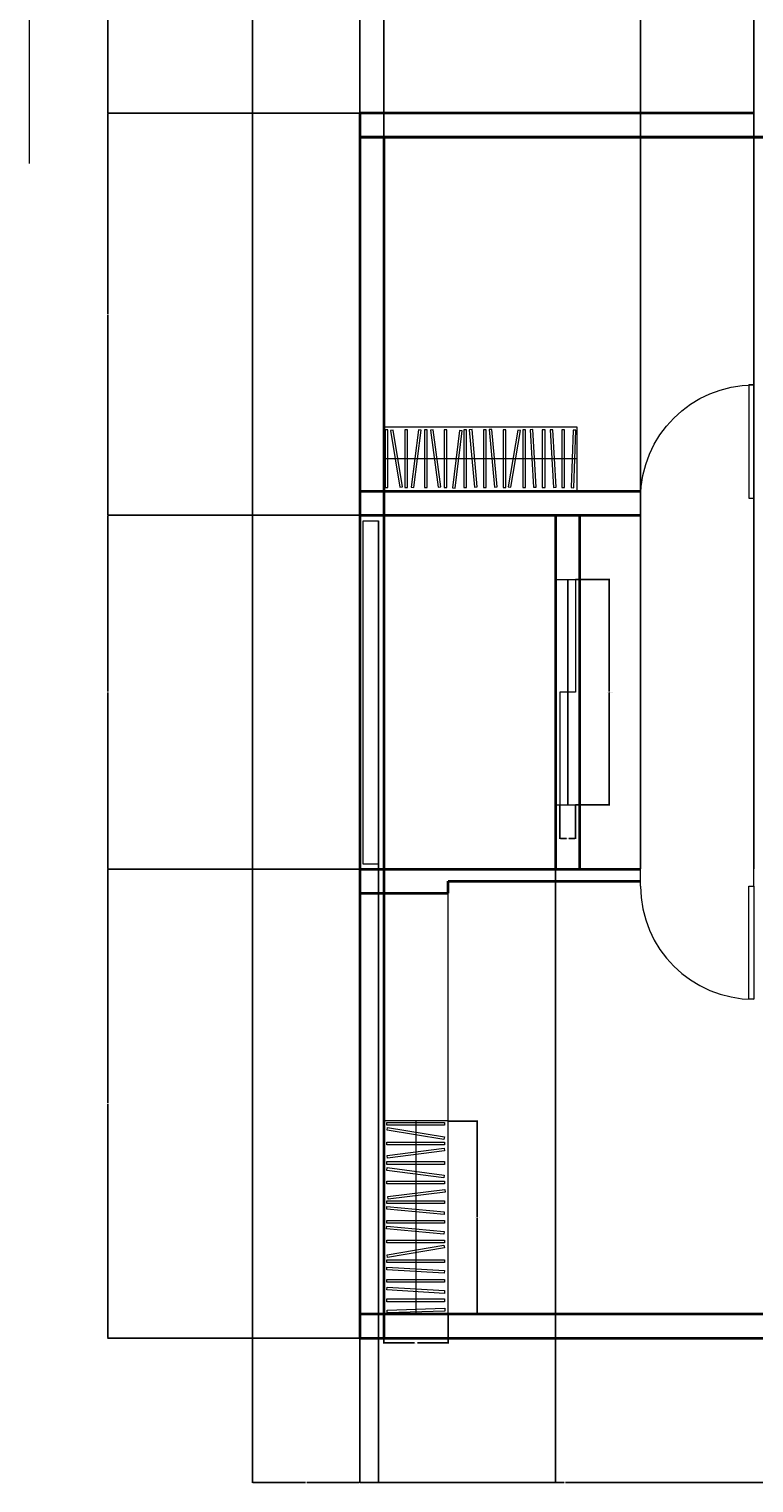
# Model space of a CAD drawing. Units: inches. Extents: x 531915 to 533151, y 849859 to 851471.
# Tile 2 of 7: x 531939 to 532210, y 850315 to 850858. Entities that reach past the tile are written whole.
import ezdxf

# ---------------------------------------------------------------- set-up
doc = ezdxf.new("R2010")
doc.units = ezdxf.units.IN
for name, color, linetype, lineweight in [('A-ANNO-DIMS', 2, 'Continuous', 18), ('A-DOOR', 3, 'Continuous', 18), ('A-FLOR-HRAL', 4, 'Continuous', 20), ('A-FURN', 8, 'Continuous', 13), ('A-WALL', 7, 'Continuous', 35)]:
    doc.layers.add(name, color=color, linetype=linetype, lineweight=lineweight)
doc.styles.get("Standard").update_dxf_attribs({"font": 'arial.ttf'})
doc.dimstyles.get("Standard").update_dxf_attribs({"dimtxt": 0.18, "dimasz": 0.18, "dimexe": 0.18, "dimexo": 0.0625, "dimgap": 0.09, "dimtad": 0, "dimtih": 1, "dimtoh": 1, "dimdec": 4, "dimzin": 0, "dimdsep": 46, "dimtxsty": 'Standard', "dimcen": 0.09, "dimadec": 0, "dimazin": 0, "dimtfac": 1, "dimtdec": 4, "dimtofl": 0, "dimtmove": 0, "dimatfit": 3, "dimfxl": 1, "dimtolj": 1, "dimtzin": 0, "dimarcsym": 0})

# ---------------------------------------------------------------- blocks, each defined once
blk = doc.blocks.new('*U2')
for p, q in [((0, 0), (0, -6)), ((40, 0), (40, -6))]:
    blk.add_line(p, q)
blk.add_lwpolyline([(0, 0), (0, 40), (1.75, 40), (1.75, 0)], close=True)
blk.add_arc((0, 0), 40, 0, 90)
blk = doc.blocks.new('WARDROBE-72')
blk.add_line((12, 0), (12, 72))
for points in [[(24, 0), (24, 72), (0, 72), (0, 0)], [(1.15, 70.47), (1.15, 71.48), (22.64, 71.48), (22.64, 70.47)], [(1.21, 68.56), (1.37, 69.55), (22.58, 66.07), (22.41, 65.07)], [(1.15, 63.15), (1.15, 64.16), (22.64, 64.16), (22.64, 63.15)], [(1.3, 58.13), (1.17, 59.13), (22.48, 61.86), (22.61, 60.86)], [(1.11, 53.59), (1.24, 54.59), (22.54, 51.79), (22.41, 50.79)], [(1.15, 55.83), (1.15, 56.84), (22.64, 56.84), (22.64, 55.83)], [(1.15, 48.51), (1.15, 49.52), (22.64, 49.52), (22.64, 48.51)], [(1.55, 42.84), (1.42, 43.84), (22.76, 46.42), (22.88, 45.42)], [(1.04, 39.13), (1.13, 40.14), (22.52, 38.16), (22.43, 37.15)], [(1.15, 41.19), (1.15, 42.2), (22.64, 42.2), (22.64, 41.19)], [(0.98, 31.76), (1.07, 32.76), (22.47, 30.78), (22.37, 29.78)], [(1.15, 33.87), (1.15, 34.88), (22.64, 34.88), (22.64, 33.87)], [(1.15, 26.55), (1.15, 27.56), (22.64, 27.56), (22.64, 26.55)], [(1.38, 21.1), (1.21, 22.1), (22.4, 25.68), (22.57, 24.68)], [(1.05, 16.46), (1.11, 17.47), (22.56, 16.21), (22.5, 15.2)], [(1.15, 19.23), (1.15, 20.24), (22.64, 20.24), (22.64, 19.23)], [(1.15, 11.91), (1.15, 12.92), (22.64, 12.92), (22.64, 11.91)], [(1.11, 8.97), (1.17, 9.98), (22.62, 8.71), (22.56, 7.7)], [(1.15, 4.59), (1.15, 5.6), (22.64, 5.6), (22.64, 4.59)], [(1.25, 0.42), (1.22, 1.43), (22.7, 2.11), (22.73, 1.1)]]:
    blk.add_lwpolyline(points, close=True)
blk = doc.blocks.new('BALCONY-SLIDER-84')
blk.add_line((2.88, 84), (2.88, 0))
for points in [[(2.88, 84), (5.76, 84), (5.76, 41.94), (2.88, 41.94)], [(2.88, 41.94), (0, 41.94), (0, 0), (2.88, 0)]]:
    blk.add_lwpolyline(points, close=True)
blk = doc.blocks.new('*D15')
at = {"layer": 'A-ANNO-DIMS', "color": 0, "lineweight": -2, "transparency": 16777216}
for p, q in [((532095.87, 850450.37), (532106.78, 850450.37)), ((532106.6, 850450.19), (532106.6, 850414.56)), ((532106.6, 850378.55), (532106.6, 850414.19)), ((532095.87, 850378.37), (532106.78, 850378.37))]:
    blk.add_line(p, q, dxfattribs=at)
at = {"layer": 'A-ANNO-DIMS', "color": 0, "transparency": 16777216}
for points in [[(532106.57, 850450.19), (532106.63, 850450.19), (532106.6, 850450.37)], [(532106.57, 850378.55), (532106.63, 850378.55), (532106.6, 850378.37)]]:
    blk.add_solid(points, dxfattribs=at)
at = {"layer": 'Defpoints', "color": 0, "transparency": 16777216}
for p in [(532095.8, 850450.37), (532106.6, 850450.37), (532095.8, 850378.37)]:
    blk.add_point(p, dxfattribs=at)
at = {"layer": 'A-ANNO-DIMS', "color": 0, "transparency": 16777216, "insert": (532106.6, 850414.37), "char_height": 0.18, "attachment_point": 5}
blk.add_mtext('\\A1;WARDROBE 72 TYP.', dxfattribs=at)
blk = doc.blocks.new('*D16')
at = {"layer": 'A-ANNO-DIMS', "color": 0, "lineweight": -2, "transparency": 16777216}
for p, q in [((532071.8, 850378.31), (532071.8, 850367.39)), ((532095.8, 850378.31), (532095.8, 850367.39)), ((532071.98, 850367.57), (532083.28, 850367.57)), ((532095.62, 850367.57), (532084.33, 850367.57))]:
    blk.add_line(p, q, dxfattribs=at)
at = {"layer": 'A-ANNO-DIMS', "color": 0, "transparency": 16777216}
for points in [[(532071.98, 850367.6), (532071.98, 850367.54), (532071.8, 850367.57)], [(532095.62, 850367.6), (532095.62, 850367.54), (532095.8, 850367.57)]]:
    blk.add_solid(points, dxfattribs=at)
at = {"layer": 'Defpoints', "color": 0, "transparency": 16777216}
for p in [(532071.8, 850378.37), (532095.8, 850378.37), (532095.8, 850367.57)]:
    blk.add_point(p, dxfattribs=at)
at = {"layer": 'A-ANNO-DIMS', "color": 0, "transparency": 16777216, "insert": (532083.8, 850367.57), "char_height": 0.18, "attachment_point": 5}
blk.add_mtext('\\A1;24 TYP.', dxfattribs=at)
blk = doc.blocks.new('*D29')
at = {"layer": 'A-ANNO-DIMS', "color": 0, "lineweight": -2, "transparency": 16777216}
for p, q in [((532143.29, 850652.37), (532156.01, 850652.37)), ((532155.83, 850652.19), (532155.83, 850610.56)), ((532155.83, 850568.55), (532155.83, 850610.19)), ((532143.29, 850568.37), (532156.01, 850568.37))]:
    blk.add_line(p, q, dxfattribs=at)
at = {"layer": 'A-ANNO-DIMS', "color": 0, "transparency": 16777216}
for points in [[(532155.8, 850652.19), (532155.86, 850652.19), (532155.83, 850652.37)], [(532155.8, 850568.55), (532155.86, 850568.55), (532155.83, 850568.37)]]:
    blk.add_solid(points, dxfattribs=at)
at = {"layer": 'Defpoints', "color": 0, "transparency": 16777216}
for p in [(532143.23, 850652.37), (532155.83, 850652.37), (532143.23, 850568.37)]:
    blk.add_point(p, dxfattribs=at)
at = {"layer": 'A-ANNO-DIMS', "color": 0, "transparency": 16777216, "insert": (532155.83, 850610.37), "char_height": 0.18, "attachment_point": 5}
blk.add_mtext('\\A1;BALCONY SLIDER 84 TYP.', dxfattribs=at)
blk = doc.blocks.new('*D30')
at = {"layer": 'A-ANNO-DIMS', "color": 0, "lineweight": -2, "transparency": 16777216}
for p, q in [((532137.47, 850568.31), (532137.47, 850555.59)), ((532143.23, 850568.31), (532143.23, 850555.59)), ((532137.65, 850555.77), (532139.89, 850555.77)), ((532143.05, 850555.77), (532140.81, 850555.77))]:
    blk.add_line(p, q, dxfattribs=at)
at = {"layer": 'A-ANNO-DIMS', "color": 0, "transparency": 16777216}
for points in [[(532137.65, 850555.8), (532137.65, 850555.74), (532137.47, 850555.77)], [(532143.05, 850555.8), (532143.05, 850555.74), (532143.23, 850555.77)]]:
    blk.add_solid(points, dxfattribs=at)
at = {"layer": 'Defpoints', "color": 0, "transparency": 16777216}
for p in [(532137.47, 850568.37), (532143.23, 850568.37), (532143.23, 850555.77)]:
    blk.add_point(p, dxfattribs=at)
at = {"layer": 'A-ANNO-DIMS', "color": 0, "transparency": 16777216, "insert": (532140.35, 850555.77), "char_height": 0.18, "attachment_point": 5}
blk.add_mtext('\\A1;6 TYP.', dxfattribs=at)
blk = doc.blocks.new('*D41')
at = {"layer": 'A-ANNO-DIMS', "color": 0, "lineweight": -2, "transparency": 16777216}
for p, q in [((532451.74, 850922.23), (531968.71, 850922.23)), ((531968.89, 850922.05), (531968.89, 850874.49)), ((531968.89, 850826.55), (531968.89, 850874.12)), ((532062.74, 850826.37), (531968.71, 850826.37))]:
    blk.add_line(p, q, dxfattribs=at)
at = {"layer": 'A-ANNO-DIMS', "color": 0, "transparency": 16777216}
for points in [[(531968.86, 850922.05), (531968.92, 850922.05), (531968.89, 850922.23)], [(531968.86, 850826.55), (531968.92, 850826.55), (531968.89, 850826.37)]]:
    blk.add_solid(points, dxfattribs=at)
at = {"layer": 'Defpoints', "color": 0, "transparency": 16777216}
for p in [(532451.8, 850922.23), (531968.89, 850826.37), (532062.8, 850826.37)]:
    blk.add_point(p, dxfattribs=at)
at = {"layer": 'A-ANNO-DIMS', "color": 0, "transparency": 16777216, "insert": (531968.89, 850874.3), "char_height": 0.18, "attachment_point": 5}
blk.add_mtext('\\A1;95.86', dxfattribs=at)
blk = doc.blocks.new('*D46')
at = {"layer": 'A-ANNO-DIMS', "color": 0, "lineweight": -2, "transparency": 16777216}
for p, q in [((532022.8, 850946.31), (532022.8, 850315.34)), ((532062.8, 850826.31), (532062.8, 850315.34)), ((532022.98, 850315.52), (532042.58, 850315.52)), ((532062.62, 850315.52), (532043.03, 850315.52))]:
    blk.add_line(p, q, dxfattribs=at)
at = {"layer": 'A-ANNO-DIMS', "color": 0, "transparency": 16777216}
for points in [[(532022.98, 850315.55), (532022.98, 850315.49), (532022.8, 850315.52)], [(532062.62, 850315.55), (532062.62, 850315.49), (532062.8, 850315.52)]]:
    blk.add_solid(points, dxfattribs=at)
at = {"layer": 'Defpoints', "color": 0, "transparency": 16777216}
for p in [(532022.8, 850946.37), (532062.8, 850826.37), (532062.8, 850315.52)]:
    blk.add_point(p, dxfattribs=at)
at = {"layer": 'A-ANNO-DIMS', "color": 0, "transparency": 16777216, "insert": (532042.8, 850315.52), "char_height": 0.18, "attachment_point": 5}
blk.add_mtext('\\A1;40', dxfattribs=at)
blk = doc.blocks.new('*D60')
at = {"layer": 'A-ANNO-DIMS', "color": 0, "lineweight": -2, "transparency": 16777216}
for p, q in [((532062.8, 850369.31), (532062.8, 850315.34)), ((532215.8, 850369.31), (532215.8, 850315.34)), ((532062.98, 850315.52), (532139.02, 850315.52)), ((532215.62, 850315.52), (532139.59, 850315.52))]:
    blk.add_line(p, q, dxfattribs=at)
at = {"layer": 'A-ANNO-DIMS', "color": 0, "transparency": 16777216}
for points in [[(532062.98, 850315.55), (532062.98, 850315.49), (532062.8, 850315.52)], [(532215.62, 850315.55), (532215.62, 850315.49), (532215.8, 850315.52)]]:
    blk.add_solid(points, dxfattribs=at)
at = {"layer": 'Defpoints', "color": 0, "transparency": 16777216}
for p in [(532062.8, 850369.37), (532215.8, 850369.37), (532215.8, 850315.52)]:
    blk.add_point(p, dxfattribs=at)
at = {"layer": 'A-ANNO-DIMS', "color": 0, "transparency": 16777216, "insert": (532139.3, 850315.52), "char_height": 0.18, "attachment_point": 5}
blk.add_mtext('\\A1;153', dxfattribs=at)
blk = doc.blocks.new('*D63')
at = {"layer": 'A-ANNO-DIMS', "color": 0, "lineweight": -2, "transparency": 16777216}
for p, q in [((532062.74, 850826.37), (531968.71, 850826.37)), ((531968.89, 850826.19), (531968.89, 850751.56)), ((531968.89, 850676.55), (531968.89, 850751.19)), ((532062.74, 850676.37), (531968.71, 850676.37))]:
    blk.add_line(p, q, dxfattribs=at)
at = {"layer": 'A-ANNO-DIMS', "color": 0, "transparency": 16777216}
for points in [[(531968.86, 850826.19), (531968.92, 850826.19), (531968.89, 850826.37)], [(531968.86, 850676.55), (531968.92, 850676.55), (531968.89, 850676.37)]]:
    blk.add_solid(points, dxfattribs=at)
at = {"layer": 'Defpoints', "color": 0, "transparency": 16777216}
for p in [(532062.8, 850826.37), (531968.89, 850676.37), (532062.8, 850676.37)]:
    blk.add_point(p, dxfattribs=at)
at = {"layer": 'A-ANNO-DIMS', "color": 0, "transparency": 16777216, "insert": (531968.89, 850751.37), "char_height": 0.18, "attachment_point": 5}
blk.add_mtext('\\A1;150', dxfattribs=at)
blk = doc.blocks.new('*D64')
at = {"layer": 'A-ANNO-DIMS', "color": 0, "lineweight": -2, "transparency": 16777216}
for p, q in [((532062.74, 850676.37), (531968.71, 850676.37)), ((531968.89, 850676.19), (531968.89, 850610.56)), ((531968.89, 850544.55), (531968.89, 850610.19)), ((532062.74, 850544.37), (531968.71, 850544.37))]:
    blk.add_line(p, q, dxfattribs=at)
at = {"layer": 'A-ANNO-DIMS', "color": 0, "transparency": 16777216}
for points in [[(531968.86, 850676.19), (531968.92, 850676.19), (531968.89, 850676.37)], [(531968.86, 850544.55), (531968.92, 850544.55), (531968.89, 850544.37)]]:
    blk.add_solid(points, dxfattribs=at)
at = {"layer": 'Defpoints', "color": 0, "transparency": 16777216}
for p in [(532062.8, 850676.37), (531968.89, 850544.37), (532062.8, 850544.37)]:
    blk.add_point(p, dxfattribs=at)
at = {"layer": 'A-ANNO-DIMS', "color": 0, "transparency": 16777216, "insert": (531968.89, 850610.37), "char_height": 0.18, "attachment_point": 5}
blk.add_mtext('\\A1;132', dxfattribs=at)
blk = doc.blocks.new('*D65')
at = {"layer": 'A-ANNO-DIMS', "color": 0, "lineweight": -2, "transparency": 16777216}
for p, q in [((532062.74, 850544.37), (531968.71, 850544.37)), ((531968.89, 850544.19), (531968.89, 850457.06)), ((531968.89, 850369.55), (531968.89, 850456.69)), ((532062.74, 850369.37), (531968.71, 850369.37))]:
    blk.add_line(p, q, dxfattribs=at)
at = {"layer": 'A-ANNO-DIMS', "color": 0, "transparency": 16777216}
for points in [[(531968.86, 850544.19), (531968.92, 850544.19), (531968.89, 850544.37)], [(531968.86, 850369.55), (531968.92, 850369.55), (531968.89, 850369.37)]]:
    blk.add_solid(points, dxfattribs=at)
at = {"layer": 'Defpoints', "color": 0, "transparency": 16777216}
for p in [(532062.8, 850544.37), (531968.89, 850369.37), (532062.8, 850369.37)]:
    blk.add_point(p, dxfattribs=at)
at = {"layer": 'A-ANNO-DIMS', "color": 0, "transparency": 16777216, "insert": (531968.89, 850456.87), "char_height": 0.18, "attachment_point": 5}
blk.add_mtext('\\A1;175', dxfattribs=at)
blk = doc.blocks.new('*D66')
at = {"layer": 'A-ANNO-DIMS', "color": 0, "lineweight": -2, "transparency": 16777216}
for p, q in [((532135.8, 850676.31), (532135.8, 850315.34)), ((532069.82, 850674.18), (532069.82, 850315.34)), ((532070, 850315.52), (532102.42, 850315.52)), ((532135.62, 850315.52), (532103.21, 850315.52))]:
    blk.add_line(p, q, dxfattribs=at)
at = {"layer": 'A-ANNO-DIMS', "color": 0, "transparency": 16777216}
for points in [[(532070, 850315.55), (532070, 850315.49), (532069.82, 850315.52)], [(532135.62, 850315.55), (532135.62, 850315.49), (532135.8, 850315.52)]]:
    blk.add_solid(points, dxfattribs=at)
at = {"layer": 'Defpoints', "color": 0, "transparency": 16777216}
for p in [(532135.8, 850676.37), (532069.82, 850674.24), (532135.8, 850315.52)]:
    blk.add_point(p, dxfattribs=at)
at = {"layer": 'A-ANNO-DIMS', "color": 0, "transparency": 16777216, "insert": (532102.81, 850315.52), "char_height": 0.18, "attachment_point": 5}
blk.add_mtext('\\A1;65.98', dxfattribs=at)
blk = doc.blocks.new('*D81')
at = {"layer": 'A-ANNO-DIMS', "color": 0, "lineweight": -2, "transparency": 16777216}
for p, q in [((532062.8, 850826.44), (532062.8, 851470.96)), ((532062.98, 851470.78), (532067.16, 851470.78)), ((532071.62, 851470.78), (532067.45, 851470.78)), ((532071.8, 850817.44), (532071.8, 851470.96))]:
    blk.add_line(p, q, dxfattribs=at)
at = {"layer": 'A-ANNO-DIMS', "color": 0, "transparency": 16777216}
for points in [[(532062.98, 851470.81), (532062.98, 851470.75), (532062.8, 851470.78)], [(532071.62, 851470.81), (532071.62, 851470.75), (532071.8, 851470.78)]]:
    blk.add_solid(points, dxfattribs=at)
at = {"layer": 'Defpoints', "color": 0, "transparency": 16777216}
for p in [(532071.8, 851470.78), (532062.8, 850826.37), (532071.8, 850817.37)]:
    blk.add_point(p, dxfattribs=at)
at = {"layer": 'A-ANNO-DIMS', "color": 0, "transparency": 16777216, "insert": (532067.3, 851470.78), "char_height": 0.18, "attachment_point": 5}
blk.add_mtext('\\A1;9', dxfattribs=at)
blk = doc.blocks.new('*D86')
at = {"layer": 'A-ANNO-DIMS', "color": 0, "lineweight": -2, "transparency": 16777216}
for p, q in [((532167.55, 850544.44), (532167.55, 851470.96)), ((532167.73, 851470.78), (532188.28, 851470.78)), ((532209.62, 851470.78), (532189.08, 851470.78)), ((532209.8, 850544.44), (532209.8, 851470.96))]:
    blk.add_line(p, q, dxfattribs=at)
at = {"layer": 'A-ANNO-DIMS', "color": 0, "transparency": 16777216}
for points in [[(532167.73, 851470.81), (532167.73, 851470.75), (532167.55, 851470.78)], [(532209.62, 851470.81), (532209.62, 851470.75), (532209.8, 851470.78)]]:
    blk.add_solid(points, dxfattribs=at)
at = {"layer": 'Defpoints', "color": 0, "transparency": 16777216}
for p in [(532209.8, 851470.78), (532167.55, 850544.37), (532209.8, 850544.37)]:
    blk.add_point(p, dxfattribs=at)
at = {"layer": 'A-ANNO-DIMS', "color": 0, "transparency": 16777216, "insert": (532188.68, 851470.78), "char_height": 0.18, "attachment_point": 5}
blk.add_mtext('\\A1;42.25', dxfattribs=at)

msp = doc.modelspace()

# ---------------------------------------------------------------- linework, layer by layer
at = {"layer": 'A-DOOR'}
for p, q in [((532135.8048, 850652.374), (532144.8048, 850652.374)), ((532135.8048, 850568.374), (532144.8048, 850568.374))]:
    msp.add_line(p, q, dxfattribs=at)
at = {"layer": 'A-FLOR-HRAL'}
msp.add_lwpolyline([(532064.0957, 850674.239), (532069.8248, 850674.239), (532069.8248, 850546.2421), (532064.0957, 850546.2421)], close=True, dxfattribs=at)
at = {"layer": 'A-FURN'}
for p, q in [((531939.4832, 850892.5471), (531939.4832, 850807.5471)), ((532095.8048, 850450.374), (532095.8048, 850535.374))]:
    msp.add_line(p, q, dxfattribs=at)
at = {"layer": 'A-WALL'}
for p, q in [((532062.8048, 850826.374), (532062.8048, 850369.374)), ((532209.8048, 850826.374), (532062.8048, 850826.374)), ((532442.8048, 850817.374), (532062.8048, 850817.374)), ((532062.8048, 850817.374), (532451.8048, 850817.374)), ((532071.8048, 850817.374), (532071.8048, 850369.374)), ((532062.8048, 850685.374), (532167.637, 850685.374)), ((532062.8048, 850676.374), (532167.553, 850676.374)), ((532135.8048, 850676.374), (532135.8048, 850544.374)), ((532144.8048, 850676.374), (532144.8048, 850544.374)), ((532062.8048, 850544.374), (532167.553, 850544.374)), ((532095.8048, 850535.374), (532095.8048, 850539.874)), ((532095.8048, 850539.874), (532167.553, 850539.874)), ((532062.8048, 850535.374), (532095.8048, 850535.374)), ((532071.8048, 850535.374), (532095.8048, 850535.374)), ((532062.8048, 850378.374), (532676.8048, 850378.374)), ((532062.8048, 850369.374), (532676.8048, 850369.374))]:
    msp.add_line(p, q, dxfattribs=at)

# ---------------------------------------------------------------- block references
at = {"layer": 'A-DOOR', "xscale": -1.056294156906435, "yscale": 1.056294156906435, "zscale": 1.056294156906435}
msp.add_blockref('*U2', (532209.8048, 850682.7117), dxfattribs=at)
at = {"layer": 'A-DOOR'}
msp.add_blockref('BALCONY-SLIDER-84', (532137.4675, 850568.374), dxfattribs=at)
at = {"layer": 'A-DOOR', "xscale": 1.056294156906435, "yscale": 1.056294156906435, "zscale": 1.056294156906435, "rotation": 180}
msp.add_blockref('*U2', (532209.8048, 850538.0362), dxfattribs=at)
at = {"layer": 'A-FURN', "extrusion": (0, 0, -1), "zscale": -1, "rotation": 269.9999999995917}
msp.add_blockref('WARDROBE-72', (-532143.8048, 850709.374), dxfattribs=at)
at = {"layer": 'A-FURN'}
msp.add_blockref('WARDROBE-72', (532071.8048, 850378.374), dxfattribs=at)

# ---------------------------------------------------------------- dimensions: what is measured, and where the dimension line sits
at = {"layer": 'A-ANNO-DIMS'}
for base, p1, p2, override, picture, middle in [((532071.8048, 851470.7848), (532062.8048, 850826.374), (532071.8048, 850817.374), {"dimdec": 0, "dimlfac": 1, "dimrnd": 0, "dimzin": 0, "dimdsep": 46, "dimlunit": 2}, '*D81', (532067.3048, 851470.7848)), ((532209.8048, 851470.7848), (532167.553, 850544.374), (532209.8048, 850544.374), {"dimdec": 2, "dimlfac": 1, "dimrnd": 0, "dimzin": 0, "dimdsep": 46, "dimlunit": 2}, '*D86', (532188.6789, 851470.7848)), ((532062.8048, 850315.524), (532022.8048, 850946.374), (532062.8048, 850826.374), {"dimdec": 0, "dimlfac": 1, "dimrnd": 0, "dimzin": 0, "dimdsep": 46, "dimlunit": 2}, '*D46', (532042.8048, 850315.524)), ((532135.8048, 850315.524), (532069.8248, 850674.239), (532135.8048, 850676.374), {"dimdec": 2, "dimlfac": 1, "dimrnd": 0, "dimzin": 0, "dimdsep": 46, "dimlunit": 2}, '*D66', (532102.8148, 850315.524)), ((532215.8048, 850315.524), (532062.8048, 850369.374), (532215.8048, 850369.374), {"dimdec": 0, "dimlfac": 1, "dimrnd": 0, "dimzin": 0, "dimdsep": 46, "dimlunit": 2}, '*D60', (532139.3048, 850315.524))]:
    dim = msp.add_linear_dim(base=base, p1=p1, p2=p2, dimstyle='Standard', override=override, dxfattribs=at)
    dim.commit()
    dim.dimension.update_dxf_attribs({"geometry": picture, "text_midpoint": middle})
for base, p1, p2, override, picture, middle in [((531968.8939, 850826.374), (532451.8048, 850922.2344), (532062.8048, 850826.374), {"dimdec": 2, "dimlfac": 1, "dimrnd": 0, "dimzin": 0, "dimdsep": 46, "dimlunit": 2}, '*D41', (531968.8939, 850874.3042)), ((531968.8939, 850676.374), (532062.8048, 850826.374), (532062.8048, 850676.374), {"dimdec": 0, "dimlfac": 1, "dimrnd": 0, "dimzin": 0, "dimdsep": 46, "dimlunit": 2}, '*D63', (531968.8939, 850751.374)), ((531968.8939, 850544.374), (532062.8048, 850676.374), (532062.8048, 850544.374), {"dimdec": 0, "dimlfac": 1, "dimrnd": 0, "dimzin": 0, "dimdsep": 46, "dimlunit": 2}, '*D64', (531968.8939, 850610.374)), ((531968.8939, 850369.374), (532062.8048, 850544.374), (532062.8048, 850369.374), {"dimdec": 0, "dimlfac": 1, "dimrnd": 0, "dimzin": 0, "dimdsep": 46, "dimlunit": 2}, '*D65', (531968.8939, 850456.874))]:
    dim = msp.add_linear_dim(base=base, p1=p1, p2=p2, angle=90, dimstyle='Standard', override=override, dxfattribs=at)
    dim.commit()
    dim.dimension.update_dxf_attribs({"geometry": picture, "text_midpoint": middle})
for base, p1, p2, text, picture, middle in [((532155.8316, 850652.374), (532143.2316, 850568.374), (532143.2316, 850652.374), 'BALCONY SLIDER <> TYP.', '*D29', (532155.8316, 850610.374)), ((532106.6048, 850450.374), (532095.8048, 850378.374), (532095.8048, 850450.374), 'WARDROBE <> TYP.', '*D15', (532106.6048, 850414.374))]:
    dim = msp.add_linear_dim(base=base, p1=p1, p2=p2, angle=90, text=text, dimstyle='Standard', override={"dimdec": 0, "dimlfac": 1, "dimrnd": 0, "dimzin": 0, "dimdsep": 46, "dimlunit": 2}, dxfattribs=at)
    dim.commit()
    dim.dimension.update_dxf_attribs({"geometry": picture, "text_midpoint": middle})
for base, p1, p2, picture, middle in [((532143.2316, 850555.774), (532137.4675, 850568.374), (532143.2316, 850568.374), '*D30', (532140.3495, 850555.774)), ((532095.8048, 850367.574), (532071.8048, 850378.374), (532095.8048, 850378.374), '*D16', (532083.8048, 850367.574))]:
    dim = msp.add_linear_dim(base=base, p1=p1, p2=p2, text='<> TYP.', dimstyle='Standard', override={"dimdec": 0, "dimlfac": 1, "dimrnd": 0, "dimzin": 0, "dimdsep": 46, "dimlunit": 2}, dxfattribs=at)
    dim.commit()
    dim.dimension.update_dxf_attribs({"geometry": picture, "text_midpoint": middle})

doc.saveas('drawing.dxf')
